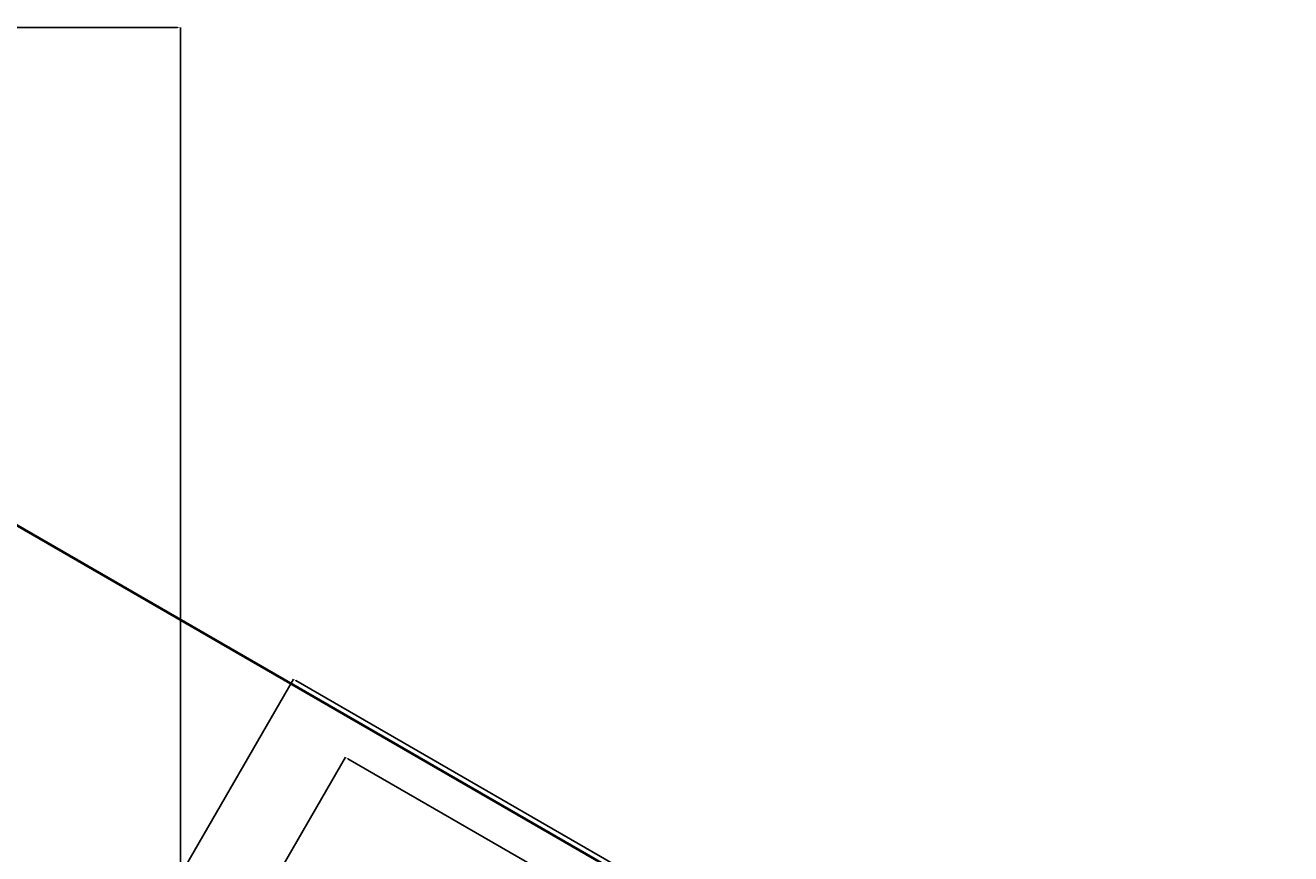
# Model space of a CAD drawing. Units: metres. Extents: x -2391 to 4922, y -635 to 4845.
# Tile 34 of 37: x 1265 to 3149, y 3611 to 4845. Entities that reach past the tile are written whole.
import ezdxf

# ---------------------------------------------------------------- set-up
doc = ezdxf.new("R2010")
doc.units = ezdxf.units.M
doc.header["$MEASUREMENT"] = 0
doc.layers.add('A-ANNO-DIMS', color=2, linetype='Continuous', lineweight=18)
doc.layers.add('A-WALL', color=7, linetype='Continuous', lineweight=50)
doc.styles.get("Standard").update_dxf_attribs({"font": 'arial.ttf'})
doc.dimstyles.get("Standard").update_dxf_attribs({"dimtxt": 5, "dimasz": 4, "dimexe": 0.18, "dimexo": 0.0625, "dimgap": 0.09, "dimtad": 0, "dimtih": 1, "dimtoh": 1, "dimdec": 0, "dimzin": 0, "dimdsep": 46, "dimtxsty": 'Standard', "dimcen": 0.09, "dimadec": 0, "dimazin": 0, "dimtfac": 1, "dimtdec": 0, "dimtofl": 0, "dimtmove": 0, "dimatfit": 3, "dimfxl": 1, "dimtolj": 1, "dimtzin": 0, "dimarcsym": 0})

# ---------------------------------------------------------------- blocks, each defined once
blk = doc.blocks.new('*D12')
at = {"layer": 'A-ANNO-DIMS', "color": 0, "lineweight": -2, "transparency": 16777216}
for p, q in [((1496.1, 3579.7), (1664.4, 3871.2)), ((1667.7, 3869), (2357.4, 3470.9)), ((3056.2, 3067.4), (2366.6, 3465.6)), ((2891.5, 2774), (3059.8, 3065.6))]:
    blk.add_line(p, q, dxfattribs=at)
at = {"layer": 'A-ANNO-DIMS', "color": 0, "transparency": 16777216}
for points in [[(1668.1, 3869.6), (1667.4, 3868.5), (1664.3, 3871)], [(3056.6, 3068), (3055.9, 3066.8), (3059.7, 3065.4)]]:
    blk.add_solid(points, dxfattribs=at)
at = {"layer": 'Defpoints', "color": 0, "transparency": 16777216}
for p in [(1496, 3579.6), (3059.7, 3065.4), (2891.4, 2774)]:
    blk.add_point(p, dxfattribs=at)
at = {"layer": 'A-ANNO-DIMS', "color": 0, "transparency": 16777216, "insert": (2362, 3468.2), "char_height": 5, "attachment_point": 5}
blk.add_mtext('\\A1;1611.3', dxfattribs=at)
blk = doc.blocks.new('*D14')
at = {"layer": 'A-ANNO-DIMS', "color": 0, "lineweight": -2, "transparency": 16777216}
for p, q in [((1573.6, 3463.3), (1741.9, 3754.8)), ((1745.2, 3752.7), (2360.9, 3397.3)), ((2985.7, 3036.5), (2370, 3392)), ((2820.9, 2743.2), (2989.2, 3034.7))]:
    blk.add_line(p, q, dxfattribs=at)
at = {"layer": 'A-ANNO-DIMS', "color": 0, "transparency": 16777216}
for points in [[(1745.6, 3753.3), (1744.9, 3752.1), (1741.8, 3754.7)], [(2986, 3037.1), (2985.3, 3036), (2989.1, 3034.5)]]:
    blk.add_solid(points, dxfattribs=at)
at = {"layer": 'Defpoints', "color": 0, "transparency": 16777216}
for p in [(1573.5, 3463.3), (2989.1, 3034.5), (2820.9, 2743.1)]:
    blk.add_point(p, dxfattribs=at)
at = {"layer": 'A-ANNO-DIMS', "color": 0, "transparency": 16777216, "insert": (2365.5, 3394.6), "char_height": 5, "attachment_point": 5}
blk.add_mtext('\\A1;1440.3', dxfattribs=at)
blk = doc.blocks.new('*D17')
at = {"layer": 'A-ANNO-DIMS', "color": 0, "lineweight": -2, "transparency": 16777216}
for p, q in [((550.7, 3005.3), (550.7, 4842)), ((554.7, 4841.8), (1014.9, 4841.8)), ((1492, 4841.8), (1031.9, 4841.8)), ((1496, 2662.5), (1496, 4842))]:
    blk.add_line(p, q, dxfattribs=at)
at = {"layer": 'A-ANNO-DIMS', "color": 0, "transparency": 16777216}
for points in [[(554.7, 4842.4), (554.7, 4841.1), (550.7, 4841.8)], [(1492, 4842.4), (1492, 4841.1), (1496, 4841.8)]]:
    blk.add_solid(points, dxfattribs=at)
at = {"layer": 'Defpoints', "color": 0, "transparency": 16777216}
for p in [(1496, 4841.8), (550.7, 3005.3), (1496, 2662.5)]:
    blk.add_point(p, dxfattribs=at)
at = {"layer": 'A-ANNO-DIMS', "color": 0, "transparency": 16777216, "insert": (1023.4, 4841.8), "char_height": 5, "attachment_point": 5}
blk.add_mtext('\\A1;945.3', dxfattribs=at)

msp = doc.modelspace()

# ---------------------------------------------------------------- linework, layer by layer
at = {"layer": 'A-WALL'}
msp.add_line((550.7419, 4505.2763), (3607.8116, 2740.2763), dxfattribs=at)

# ---------------------------------------------------------------- dimensions: what is measured, and where the dimension line sits
at = {"layer": 'A-ANNO-DIMS'}
dim = msp.add_linear_dim(base=(1496.0309, 4841.7763), p1=(550.7419, 3005.2763), p2=(1496.0309, 2662.4566), dimstyle='Standard', override={"dimdec": 1, "dimlfac": 1, "dimrnd": 0, "dimzin": 0, "dimdsep": 46, "dimlunit": 2}, dxfattribs=at)
dim.commit()
dim.dimension.update_dxf_attribs({"geometry": '*D17', "text_midpoint": (1023.3864, 4841.7763)})
for base, p1, p2, picture, middle in [((3059.6824, 3065.3977), (1496.0309, 3579.6156), (2891.4324, 2773.9801), '*D12', (2361.9817, 3468.2154)), ((2989.1268, 3034.536), (1573.5273, 3463.276), (2820.8768, 2743.1184), '*D14', (2365.4521, 3394.6148))]:
    dim = msp.add_linear_dim(base=base, p1=p1, p2=p2, angle=330, dimstyle='Standard', override={"dimdec": 1, "dimlfac": 1, "dimrnd": 0, "dimzin": 0, "dimdsep": 46, "dimlunit": 2}, dxfattribs=at)
    dim.commit()
    dim.dimension.update_dxf_attribs({"geometry": picture, "text_midpoint": middle})

doc.saveas('drawing.dxf')
